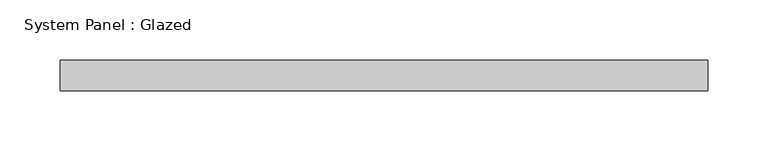
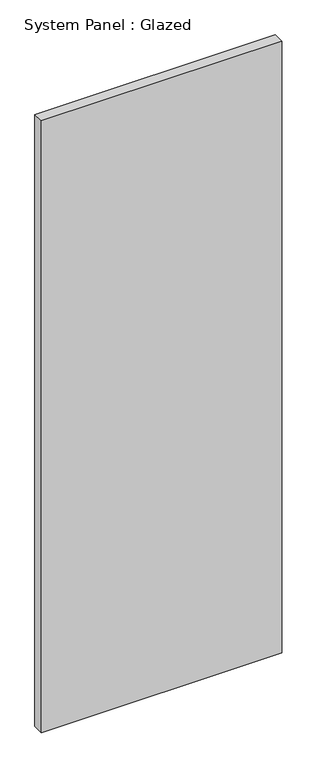
"""IFC4 building model written with IfcOpenShell, lengths in millimetres: plate geometry, System Panel : Glazed."""

from ifc_helpers import new_model, si_unit, origin, origin_with_axes, place, context, project, spatial, polyline, outline, extrude, source, transform, mapped, element, save


def system_panel_glazed_6b96ba39(model_context):
    return source(origin(), model_context, "Body", "SweptSolid", [
        extrude(outline(polyline([(269.875, 19.05), (-269.875, 19.05), (-269.875, 44.45), (269.875, 44.45), (269.875, 19.05)])), origin_with_axes(), (0.0, 0.0, 1.0), 1453.0534505),
    ])


if __name__ == "__main__":
    model = new_model("IFC4")
    model_context = context("Model", 3, world=origin())
    ifc_project = project(units=[si_unit("LENGTHUNIT", "METRE", prefix="MILLI")], contexts=[model_context])
    site = spatial("IfcSite", under=ifc_project)
    building = spatial("IfcBuilding", under=site)
    placement = place(None, origin())
    system_panel_glazed_shape = system_panel_glazed_6b96ba39(model_context)
    element("IfcPlate", 1, ObjectType="System Panel : Glazed", at=placement, inside=building, context=model_context, shape_type="MappedRepresentation", body=[
        mapped(system_panel_glazed_shape, transform((0.0, 0.0, 0.0), x_axis=(1.0, 0.0, 0.0), y_axis=(0.0, 1.0, 0.0), z_axis=(0.0, 0.0, 1.0))),
    ])
    save(model, "model.ifc")

# Revit data of these elements
# Type "System Panel : Glazed"
#   Construction Type Id = "GSP4R"
#   Analytic Construction = "1/8 in Pilkington single glazing"
#   Visual Light Transmittance = 0.9
#   Solar Heat Gain Coefficient = 0.86
#   Heat Transfer Coefficient (U) = 1.18115 BTU/(h·ft²·°F)
#   Define Thermal Properties by = 1
# Element 1 (IfcPlate, "System Panel : Glazed")
#   Materials on its faces: "Glass"
# Materials
#   "Glass": class "Glass", colour RGB 0 128 192, transparency 0.75, Description = "Soda Lime Glass", Cost = 0
